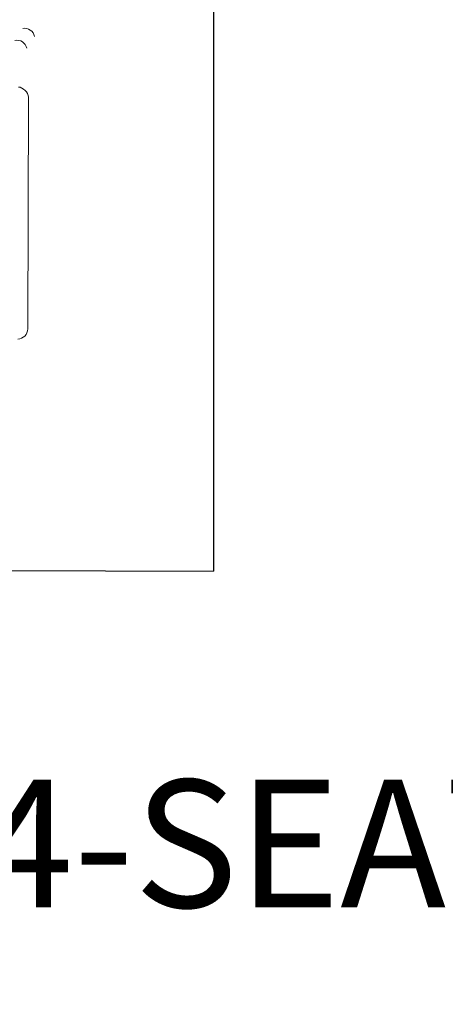
# Model space of a CAD drawing. Units: inches. Extents: x -466983 to 1020, y 324 to 318697.
# Tile 38 of 97: x 888 to 908, y 734 to 781. Entities that reach past the tile are written whole.
import ezdxf

# ---------------------------------------------------------------- set-up
doc = ezdxf.new("R2010")
doc.units = ezdxf.units.IN
doc.header["$MEASUREMENT"] = 0
for name, color, linetype, lineweight in [('A-ANNO-DIMS', 2, 'Continuous', 18), ('A-FLOR-PATT', 252, 'Continuous', 13), ('A-FURN', 8, 'Continuous', 18), ('CBV_01', 7, 'Continuous', 0)]:
    doc.layers.add(name, color=color, linetype=linetype, lineweight=lineweight)
doc.layers.add('Office Desk', color=30, linetype='Continuous', true_color=0xeb7500)
doc.styles.get("Standard").update_dxf_attribs({"font": 'arial.ttf'})
doc.dimstyles.get("Standard").update_dxf_attribs({"dimtxt": 6, "dimasz": 4, "dimexe": 3, "dimexo": 3, "dimgap": 0.09, "dimtad": 0, "dimtih": 1, "dimtoh": 1, "dimdec": 1, "dimzin": 0, "dimdsep": 46, "dimlunit": 3, "dimtxsty": 'Standard', "dimcen": 0.09, "dimadec": 0, "dimazin": 0, "dimtfac": 1, "dimtdec": 1, "dimtofl": 0, "dimtmove": 0, "dimatfit": 3, "dimfxl": 1, "dimtolj": 1, "dimtzin": 0, "dimarcsym": 0})

# ---------------------------------------------------------------- blocks, each defined once
blk = doc.blocks.new('Offce Table')
at = {"layer": 'CBV_01'}
blk.add_line((2626.919, 961.576, -0.016), (2626.948, 972.47, -0.016), dxfattribs=at)
for centre, start, end in [((2626.774, 975.233, -0.016), 11.2965, 101.2965), ((2626.403, 974.675, -0.016), 11.2965, 101.2965), ((2626.445, 961.578, -0.016), 269.8453, 359.8453)]:
    blk.add_arc(centre, 0.474, start, end, dxfattribs=at)
blk.add_open_spline([(2626.948, 972.47, -0.016), (2626.949, 972.693, -0.016), (2626.699, 972.944, -0.016), (2626.476, 972.945, -0.016)], degree=3, dxfattribs=at)
at = {"layer": 'Office Desk'}
for p in [(2635.658, 981.455, -0.016), (2575.658, 950.355, -0.016)]:
    blk.add_line(p, (2635.658, 950.194, -0.016), dxfattribs=at)
blk = doc.blocks.new('Office Desk With Chairs')
blk.add_blockref('Offce Table', (-526.404, 94.584))
blk = doc.blocks.new('*D91')
at = {"layer": 'A-ANNO-DIMS', "color": 0, "lineweight": -2, "transparency": 16777216}
for p, q in [((938.253, 802.547), (920.07, 802.547)), ((923.07, 798.547), (923.07, 745.132)), ((923.07, 685.328), (923.07, 738.743)), ((938.253, 681.328), (920.07, 681.328))]:
    blk.add_line(p, q, dxfattribs=at)
at = {"layer": 'A-ANNO-DIMS', "color": 0, "transparency": 16777216}
for points in [[(922.404, 798.547), (923.737, 798.547), (923.07, 802.547)], [(922.404, 685.328), (923.737, 685.328), (923.07, 681.328)]]:
    blk.add_solid(points, dxfattribs=at)
at = {"layer": 'Defpoints', "color": 0, "transparency": 16777216}
for p in [(941.253, 802.547), (923.07, 681.328), (941.253, 681.328)]:
    blk.add_point(p, dxfattribs=at)
at = {"layer": 'A-ANNO-DIMS', "color": 0, "transparency": 16777216, "insert": (923.07, 741.937), "char_height": 6, "attachment_point": 5}
blk.add_mtext('\\A1;4-SEATER SOFA 121', dxfattribs=at)

msp = doc.modelspace()

# ---------------------------------------------------------------- hatches: boundary and pattern name
at = {"layer": 'A-FLOR-PATT', "transparency": 33554572}
h = msp.add_hatch(dxfattribs=at)
h.set_pattern_fill('ANSI37', color=256, scale=30)
h.set_pattern_definition([(45, (-1212.4137, -290.035), (-2.6516504, 2.6516504), []), (135, (-1212.4137, -290.035), (-2.6516504, -2.6516504), [])])
h.paths.add_polyline_path([(901.806, 1075.938), (900.614, 1075.938), (900.614, 1065.386), (899.391, 1065.386), (898.091, 1065.386), (892.836, 1058.71, -0.258377), (892.188, 1058.351), (879.985, 1058.351, -0.20177), (879.438, 1058.581), (874.081, 1065.386), (872.781, 1065.386), (871.558, 1065.386), (871.558, 1075.938), (813.806, 1075.938), (813.806, 1044.792), (832.395, 1044.792, -0.394795), (848.66, 1028.536), (848.66, 1009.938), (901.806, 1009.938), (901.806, 1015.938), (901.306, 1015.938), (871.306, 1015.938), (871.306, 1017.25), (871.334, 1017.25, -0.401453), (901.306, 1045.938), (901.806, 1045.938)])
edge = h.paths.add_edge_path(flags=16)
edge.add_line((847.773, 1068.949), (847.773, 1073.709))
edge.add_arc((849.227, 1073.709), 1.454, 90, 180, ccw=False)
edge.add_line((849.227, 1075.163), (864.492, 1075.163))
edge.add_arc((864.492, 1073.709), 1.454, 0, 90, ccw=False)
edge.add_line((865.946, 1073.709), (865.946, 1069.004))
edge.add_arc((832.645, 1068.976), 33.301, -20.6123, 0.0472, ccw=False)
edge.add_ellipse((856.859, 1058.48), major_axis=(0, 10.213), ratio=0.685919, start_angle=100.0088, end_angle=259.9912, ccw=False)
edge.add_arc((881.074, 1068.976), 33.301, 180.0472, 200.6123, ccw=False)
h.paths.add_polyline_path([(853.146, 1066.482), (853.146, 1066.453), (853.146, 1066.453, 0.433107), (852.917, 1066.685), (852.917, 1066.453), (853.146, 1066.453), (853.146, 1066.482), (853.088, 1066.612, 0.697939), (852.7, 1066.453), (852.7, 1066.453), (852.7, 1066.482), (852.917, 1067.001), (852.917, 1066.685, -0.396254)], flags=0)
h.paths.add_polyline_path([(861.019, 1066.482), (861.019, 1066.453), (861.019, 1066.453, 0.416404), (860.802, 1066.685), (860.802, 1066.453), (861.019, 1066.453), (861.019, 1066.482), (860.967, 1066.605, 0.713344), (860.573, 1066.453), (860.573, 1066.453), (860.573, 1066.482), (860.802, 1067.001), (860.802, 1066.685, -0.379973)], flags=0)
edge = h.paths.add_edge_path(flags=0)
edge.add_spline(control_points=[(861.13, 1065.785), (861.466, 1065.248), (861.613, 1065.016), (861.983, 1064.374), (862.192, 1063.944), (862.561, 1063.039), (862.721, 1062.563), (862.987, 1061.578), (863.092, 1061.069), (863.245, 1060.031), (863.293, 1059.503), (863.329, 1058.441), (863.318, 1057.908), (863.237, 1056.852), (863.166, 1056.329), (862.97, 1055.308), (862.843, 1054.81), (862.537, 1053.852), (862.357, 1053.393), (861.951, 1052.525), (861.725, 1052.117), (861.233, 1051.362), (860.967, 1051.016), (860.405, 1050.395), (860.108, 1050.12), (859.494, 1049.646), (859.176, 1049.448), (858.528, 1049.13), (858.197, 1049.011), (857.531, 1048.852), (857.196, 1048.812), (856.525, 1048.812), (856.189, 1048.852), (855.524, 1049.01), (855.193, 1049.129), (854.545, 1049.447), (854.227, 1049.645), (853.612, 1050.118), (853.316, 1050.393), (852.753, 1051.014), (852.487, 1051.36), (851.995, 1052.114), (851.769, 1052.523), (851.363, 1053.39), (851.183, 1053.85), (850.877, 1054.807), (850.75, 1055.305), (850.553, 1056.326), (850.483, 1056.849), (850.401, 1057.905), (850.39, 1058.438), (850.426, 1059.5), (850.473, 1060.028), (850.626, 1061.066), (850.732, 1061.575), (850.997, 1062.561), (851.157, 1063.036), (851.525, 1063.942), (851.734, 1064.371), (852.106, 1065.016), (852.254, 1065.25), (852.608, 1065.733)], knot_values=[3.915332, 3.915332, 3.915332, 3.915332, 4.013468, 4.013468, 4.175532, 4.175532, 4.337596, 4.337596, 4.49966, 4.49966, 4.661724, 4.661724, 4.823788, 4.823788, 4.985852, 4.985852, 5.147916, 5.147916, 5.30998, 5.30998, 5.472044, 5.472044, 5.634109, 5.634109, 5.796173, 5.796173, 5.958237, 5.958237, 6.120301, 6.120301, 6.282365, 6.282365, 6.444429, 6.444429, 6.606493, 6.606493, 6.768557, 6.768557, 6.930621, 6.930621, 7.092685, 7.092685, 7.254749, 7.254749, 7.416813, 7.416813, 7.578878, 7.578878, 7.740942, 7.740942, 7.903006, 7.903006, 8.06507, 8.06507, 8.227134, 8.227134, 8.389198, 8.389198, 8.551262, 8.551262, 8.65037, 8.65037, 8.65037, 8.65037], degree=3, periodic=0)
edge.add_line((852.642, 1065.785), (861.13, 1065.785))
edge = h.paths.add_edge_path(flags=0)
edge.add_ellipse((856.85, 1057.743), major_axis=(0, 7.792), ratio=0.687861, start_angle=0, end_angle=360)
h.paths.add_polyline_path([(848.863, 1069.389), (848.863, 1073.96, -0.414214), (849.954, 1075.051), (863.765, 1075.051, -0.414214), (864.856, 1073.96), (864.856, 1069.389, -0.388936), (864.524, 1069.027, -0.043561), (849.195, 1069.027, -0.388936)], flags=0)
h.paths.add_polyline_path([(853.101, 1068.112, -1), (852.677, 1068.112, -1)], flags=0)
edge = h.paths.add_edge_path(flags=0)
edge.add_ellipse((856.859, 1057.338), major_axis=(0, 2.207), ratio=0.657164, start_angle=0, end_angle=360)
h.paths.add_polyline_path([(861.041, 1068.112, -1), (860.618, 1068.112, -1)], flags=0)
edge = h.paths.add_edge_path()
edge.add_line((573.954, 1057.341), (573.954, 1075.938))
edge.add_line((573.954, 1075.938), (558.731, 1075.938))
edge.add_line((558.731, 1075.938), (558.731, 1065.386))
edge.add_line((558.731, 1065.386), (557.507, 1065.386))
edge.add_line((557.507, 1065.386), (556.207, 1065.386))
edge.add_line((556.207, 1065.386), (550.952, 1058.71))
edge.add_arc((550.304, 1059.116), 0.765, 270, 327.9483, ccw=False)
edge.add_line((550.304, 1058.351), (538.101, 1058.351))
edge.add_arc((538.101, 1059.116), 0.765, 224.3704, 270, ccw=False)
edge.add_line((537.555, 1058.581), (532.198, 1065.386))
edge.add_line((532.198, 1065.386), (530.898, 1065.386))
edge.add_line((530.898, 1065.386), (529.674, 1065.386))
edge.add_line((529.674, 1065.386), (529.674, 1075.938))
edge.add_line((529.674, 1075.938), (520.806, 1075.938))
edge.add_line((520.806, 1075.938), (520.806, 1045.938))
edge.add_line((520.806, 1045.938), (521.306, 1045.938))
edge.add_arc((521.306, 1015.938), 30, 2.5075, 90, ccw=False)
edge.add_line((551.277, 1017.25), (551.306, 1017.25))
edge.add_line((551.306, 1017.25), (551.306, 1015.938))
edge.add_line((551.306, 1015.938), (520.806, 1015.938))
edge.add_line((520.806, 1015.938), (520.806, 1009.938))
edge.add_line((520.806, 1009.938), (559.191, 1010.402))
edge.add_arc((559.191, 1011.856), 1.454, 180, 270, ccw=False)
edge.add_line((557.737, 1011.856), (557.737, 1016.561))
edge.add_arc((591.039, 1016.589), 33.301, 159.3877, 180.0472, ccw=False)
edge.add_ellipse((566.824, 1027.085), major_axis=(0, 10.213), ratio=0.685919, start_angle=280.0088, end_angle=439.9912, ccw=False)
edge.add_arc((542.609, 1016.589), 33.301, 0.0472, 20.6123, ccw=False)
edge.add_line((575.91, 1016.616), (575.91, 1011.856))
edge.add_arc((574.456, 1011.856), 1.454, -90, 0, ccw=False)
edge.add_line((574.456, 1010.402), (608.806, 1009.938))
edge.add_line((608.806, 1009.938), (608.806, 1041.086))
edge.add_line((608.806, 1041.086), (590.218, 1041.086))
edge.add_arc((590.775, 1057.907), 16.831, 181.9277, 268.1032, ccw=False)
edge = h.paths.add_edge_path()
edge.add_ellipse((494.244, 583.62), major_axis=(0, 10.213), ratio=0.685919, start_angle=280.0088, end_angle=439.9912, ccw=False)
edge.add_arc((470.03, 573.124), 33.301, 0.0472, 20.6123, ccw=False)
edge.add_line((503.331, 573.152), (503.331, 568.392))
edge.add_arc((501.877, 568.392), 1.454, -90, 0, ccw=False)
edge.add_line((501.877, 566.938), (539.806, 566.938))
edge.add_line((539.806, 566.938), (539.806, 572.938))
edge.add_line((539.806, 572.938), (539.306, 572.938))
edge.add_line((539.306, 572.938), (509.306, 572.938))
edge.add_line((509.306, 572.938), (509.306, 574.25))
edge.add_line((509.306, 574.25), (509.334, 574.25))
edge.add_arc((539.306, 572.938), 30, 90, 177.4925, ccw=False)
edge.add_line((539.306, 602.938), (539.806, 602.938))
edge.add_line((539.806, 602.938), (539.806, 626.938))
edge.add_line((539.806, 626.938), (531.772, 626.938))
edge.add_line((531.772, 626.938), (531.772, 616.386))
edge.add_line((531.772, 616.386), (530.548, 616.386))
edge.add_line((530.548, 616.386), (529.249, 616.386))
edge.add_line((529.249, 616.386), (523.711, 609.351))
edge.add_line((523.711, 609.351), (510.777, 609.351))
edge.add_line((510.777, 609.351), (505.239, 616.386))
edge.add_line((505.239, 616.386), (503.939, 616.386))
edge.add_line((503.939, 616.386), (502.715, 616.386))
edge.add_line((502.715, 616.386), (502.715, 626.938))
edge.add_line((502.715, 626.938), (481.698, 626.938))
edge.add_line((481.698, 626.938), (481.698, 610.995))
edge.add_arc((467.27, 611.473), 14.436, 271.9277, 358.1032, ccw=False)
edge.add_line((467.756, 597.045), (451.806, 597.045))
edge.add_line((451.806, 597.045), (451.806, 584.404))
edge.add_line((451.806, 584.404), (451.806, 566.938))
edge.add_line((451.806, 566.938), (486.612, 566.938))
edge.add_arc((486.612, 568.392), 1.454, 180, 270, ccw=False)
edge.add_line((485.158, 568.392), (485.158, 573.097))
edge.add_arc((518.459, 573.124), 33.301, 159.3877, 180.0472, ccw=False)
h.paths.add_polyline_path([(836.261, 1020.733), (879.89, 1020.733), (879.89, 1039.39), (836.261, 1039.39)], flags=25)
h.paths.add_polyline_path([(549.985, 1036.749), (593.614, 1036.749), (593.614, 1055.407), (549.985, 1055.407)], flags=24)
h.paths.add_polyline_path([(475.123, 595.596), (518.752, 595.596), (518.752, 614.253), (475.123, 614.253)], flags=24)

# ---------------------------------------------------------------- block references
at = {"layer": 'A-FURN'}
msp.add_blockref('Office Desk With Chairs', (-1212.414, -290.035), dxfattribs=at)

# ---------------------------------------------------------------- dimensions: what is measured, and where the dimension line sits
at = {"layer": 'A-ANNO-DIMS'}
dim = msp.add_linear_dim(base=(923.07, 681.328), p1=(941.253, 802.547), p2=(941.253, 681.328), angle=270, text='4-SEATER SOFA <>', dimstyle='Standard', override={"dimdec": 0, "dimlfac": 1, "dimrnd": 0, "dimzin": 0, "dimdsep": 46, "dimlunit": 2}, dxfattribs=at)
dim.commit()
dim.dimension.update_dxf_attribs({"geometry": '*D91', "text_midpoint": (923.07, 741.937)})

doc.saveas('drawing.dxf')
